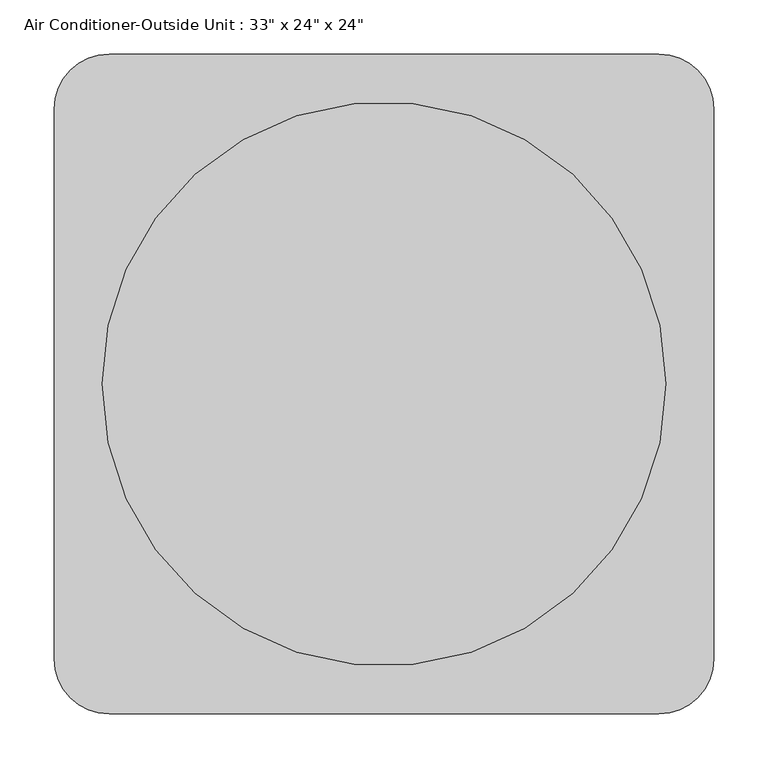
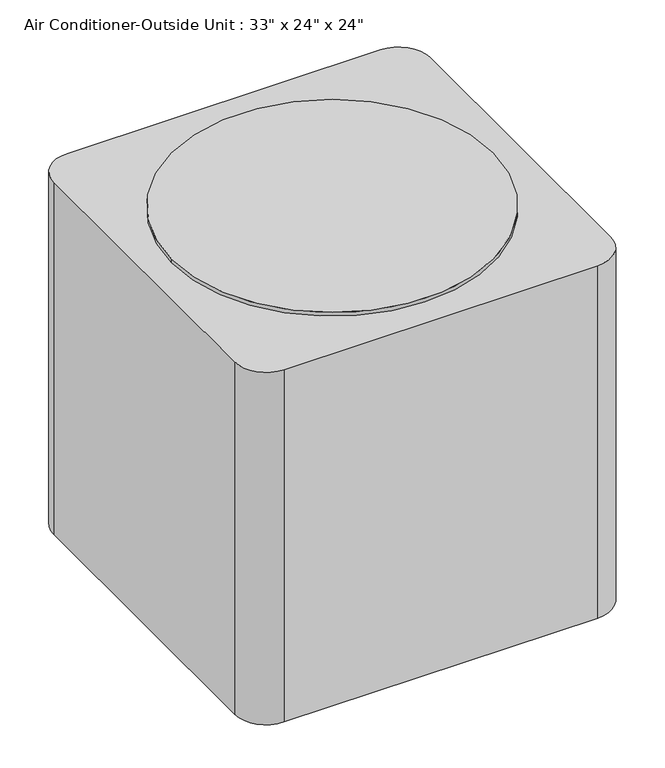
"""IFC4 building model written with IfcOpenShell, lengths in millimetres: proxy geometry."""

from ifc_helpers import new_model, si_unit, point, frame, frame_2d, origin, origin_with_axes, origin_2d, place, context, project, spatial, polyline, circle_curve, trimmed, segment, composite_curve, outline, extrude, source, transform, mapped, element, save


def proxy_13b82c07(model_context):
    return source(origin(), model_context, "Body", "SweptSolid", [
        extrude(outline(composite_curve([segment(trimmed(circle_curve(origin_2d(), 260.4633699), [point((-260.4633699, 0.0))], [point((260.4633699, 0.0))], False, "CARTESIAN"), True, "CONTINUOUS"), segment(trimmed(circle_curve(origin_2d(), 260.4633699), [point((260.4633699, 0.0))], [point((-260.4633699, 0.0))], False, "CARTESIAN"), True, "CONTINUOUS")], self_intersect=False)), frame((0.0, 0.0, 603.25), z_axis=(0.0, 0.0, 1.0), x_axis=(1.0, 0.0, 0.0)), (0.0, 0.0, 1.0), 6.35),
        extrude(outline(composite_curve([segment(polyline([(254.0, -304.8), (-254.0, -304.8)]), True, "CONTINUOUS"), segment(trimmed(circle_curve(frame_2d((-254.0, -254.0)), 50.8), [point((-254.0, -304.8))], [point((-304.8, -254.0))], False, "CARTESIAN"), True, "CONTINUOUS"), segment(polyline([(-304.8, -254.0), (-304.8, 254.0)]), True, "CONTINUOUS"), segment(trimmed(circle_curve(frame_2d((-254.0, 254.0)), 50.8), [point((-304.8, 254.0))], [point((-254.0, 304.8))], False, "CARTESIAN"), True, "CONTINUOUS"), segment(polyline([(-254.0, 304.8), (254.0, 304.8)]), True, "CONTINUOUS"), segment(trimmed(circle_curve(frame_2d((254.0, 254.0)), 50.8), [point((254.0, 304.8))], [point((304.8, 254.0))], False, "CARTESIAN"), True, "CONTINUOUS"), segment(polyline([(304.8, 254.0), (304.8, -254.0)]), True, "CONTINUOUS"), segment(trimmed(circle_curve(frame_2d((254.0, -254.0)), 50.8), [point((304.8, -254.0))], [point((254.0, -304.8))], False, "CARTESIAN"), True, "CONTINUOUS")], self_intersect=False)), origin_with_axes(), (0.0, 0.0, 1.0), 603.25),
    ])


if __name__ == "__main__":
    model = new_model("IFC4")
    model_context = context("Model", 3, world=origin())
    ifc_project = project(units=[si_unit("LENGTHUNIT", "METRE", prefix="MILLI")], contexts=[model_context])
    site = spatial("IfcSite", under=ifc_project)
    building = spatial("IfcBuilding", under=site)
    placement = place(None, origin())
    proxy_shape = proxy_13b82c07(model_context)
    element("IfcBuildingElementProxy", 1, Name="Air Conditioner-Outside Unit : 33\" x 24\" x 24\"", ObjectType="Air Conditioner-Outside Unit : 33\" x 24\" x 24\"", at=placement, inside=building, context=model_context, shape_type="MappedRepresentation", body=[
        mapped(proxy_shape, transform((0.0, 0.0, 0.0), x_axis=(1.0, 0.0, 0.0), y_axis=(0.0, 1.0, 0.0), z_axis=(0.0, 0.0, 1.0))),
    ])
    save(model, "model.ifc")

# Revit data of these elements
# Type "Air Conditioner-Outside Unit : 33\" x 24\" x 24\""
#   Assembly Code = "D3030"
#   Depth = 2' - 0"
#   Height = 2' - 0"
#   Width = 2' - 0"
#   Air Conditioner Material = Steel, Paint Finish, Dark Gray, Matte
#   Default Elevation = 0
# Element 1 (IfcBuildingElementProxy, "Air Conditioner-Outside Unit : 33\" x 24\" x 24\"")
#   Materials on its faces: "Steel, Paint Finish, Dark Gray, Matte"
# Materials
#   "Steel, Paint Finish, Dark Gray, Matte": class "Metal", colour RGB 98 98 98, transparency 0, Description = "Steel, paint finish, dark gray, matte", Cost = 0
